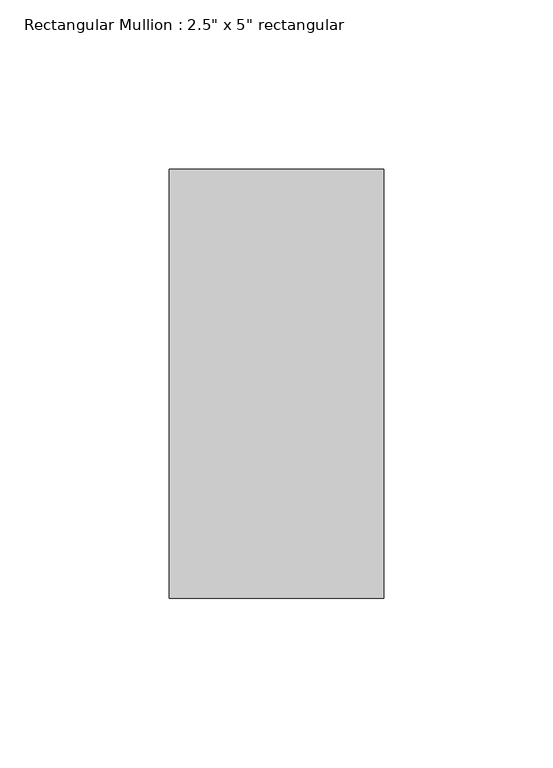
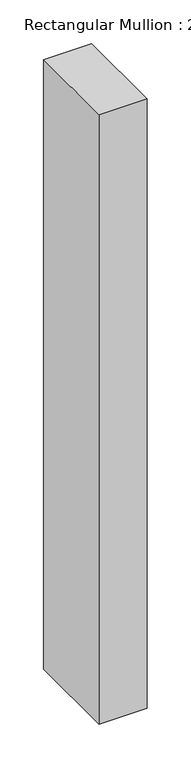
"""IFC4 building model written with IfcOpenShell, lengths in millimetres: member geometry."""

from ifc_helpers import new_model, si_unit, frame, origin, place, context, project, spatial, polyline, outline, extrude, source, transform, mapped, element, save


def member_9b18e963(model_context):
    return source(origin(), model_context, "Body", "SweptSolid", [
        extrude(outline(polyline([(0.0, 63.5), (0.0, -63.5), (-63.5, -63.5), (-63.5, 63.5), (0.0, 63.5)])), frame((0.0, 0.0, -850.8999998), z_axis=(0.0, 0.0, 1.0), x_axis=(1.0, 0.0, 0.0)), (0.0, 0.0, 1.0), 850.8999998),
    ])


if __name__ == "__main__":
    model = new_model("IFC4")
    model_context = context("Model", 3, world=origin())
    ifc_project = project(units=[si_unit("LENGTHUNIT", "METRE", prefix="MILLI")], contexts=[model_context])
    site = spatial("IfcSite", under=ifc_project)
    building = spatial("IfcBuilding", under=site)
    placement = place(None, origin())
    member_shape = member_9b18e963(model_context)
    element("IfcMember", 1, ObjectType="Rectangular Mullion : 2.5\" x 5\" rectangular", at=placement, inside=building, context=model_context, shape_type="MappedRepresentation", body=[
        mapped(member_shape, transform((0.0, 0.0, 0.0), x_axis=(1.0, 0.0, 0.0), y_axis=(0.0, 1.0, 0.0), z_axis=(0.0, 0.0, 1.0))),
    ])
    save(model, "model.ifc")

# Revit data of these elements
# Type "Rectangular Mullion : 2.5\" x 5\" rectangular"
#   built-in parameter 1007304 = 0.416667 (stored number, unit not read)
#   built-in parameter 1007301 = 0.104167 (stored number, unit not read)
#   built-in parameter 1007300 = 0.104167 (stored number, unit not read)
# Element 1 (IfcMember, "Rectangular Mullion : 2.5\" x 5\" rectangular")
#   Materials on its faces: "Aluminum"
# Materials
#   "Aluminum": class "Metal", colour RGB 247 247 247, transparency 0, Description = "Aluminum 6061", Cost = 0
